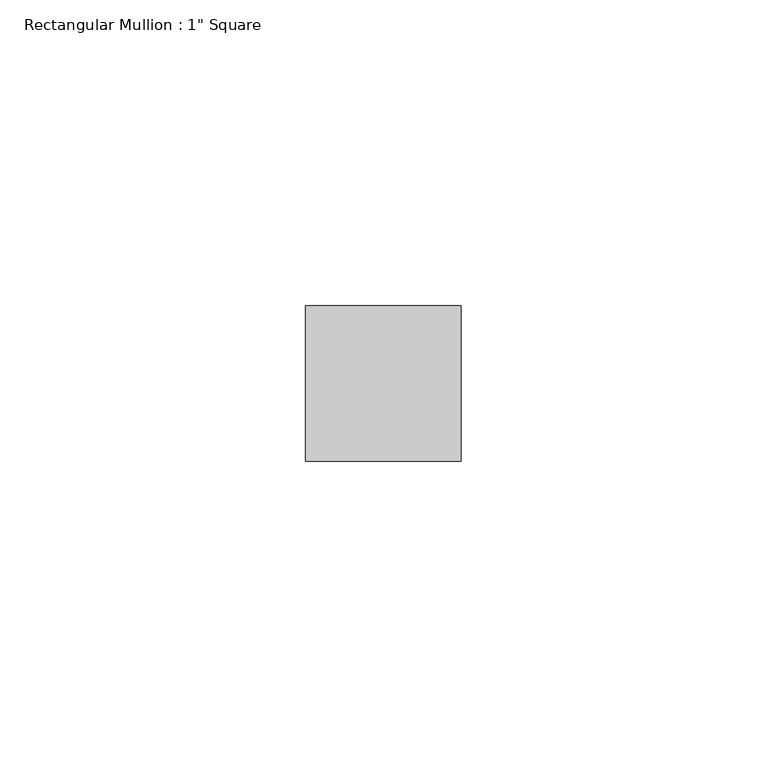
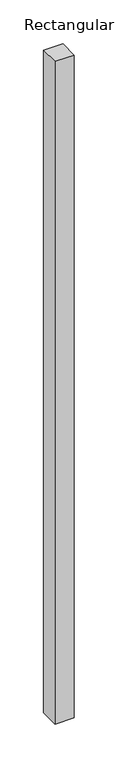
"""IFC4 building model written with IfcOpenShell, lengths in millimetres: member geometry."""

from ifc_helpers import new_model, si_unit, frame, origin, place, context, project, spatial, polyline, outline, extrude, source, transform, mapped, element, save


def member_df2e51ae(model_context):
    return source(origin(), model_context, "Body", "SweptSolid", [
        extrude(outline(polyline([(12.7, 12.7), (12.7, -12.7), (-12.7, -12.7), (-12.7, 12.7), (12.7, 12.7)])), frame((0.0, 0.0, -920.75), z_axis=(0.0, 0.0, 1.0), x_axis=(1.0, 0.0, 0.0)), (0.0, 0.0, 1.0), 920.75),
    ])


if __name__ == "__main__":
    model = new_model("IFC4")
    model_context = context("Model", 3, world=origin())
    ifc_project = project(units=[si_unit("LENGTHUNIT", "METRE", prefix="MILLI")], contexts=[model_context])
    site = spatial("IfcSite", under=ifc_project)
    building = spatial("IfcBuilding", under=site)
    placement = place(None, origin())
    member_shape = member_df2e51ae(model_context)
    element("IfcMember", 1, ObjectType="Rectangular Mullion : 1\" Square", at=placement, inside=building, context=model_context, shape_type="MappedRepresentation", body=[
        mapped(member_shape, transform((0.0, 0.0, 0.0), x_axis=(1.0, 0.0, 0.0), y_axis=(0.0, 1.0, 0.0), z_axis=(0.0, 0.0, 1.0))),
    ])
    save(model, "model.ifc")

# Revit data of these elements
# Type "Rectangular Mullion : 1\" Square"
#   built-in parameter 1007304 = 0.0833333 (stored number, unit not read)
#   built-in parameter 1007301 = 0.0416667 (stored number, unit not read)
#   built-in parameter 1007300 = 0.0416667 (stored number, unit not read)
# Element 1 (IfcMember, "Rectangular Mullion : 1\" Square")
#   Materials on its faces: "Rectangle 1 sq"
# Materials
#   "Rectangle 1 sq": class "Generic", colour RGB 120 120 120, transparency 0, Cost = 0
